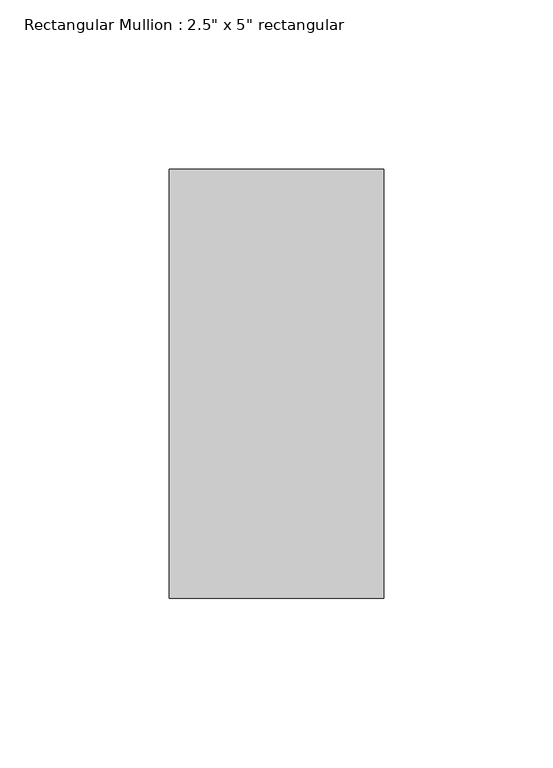
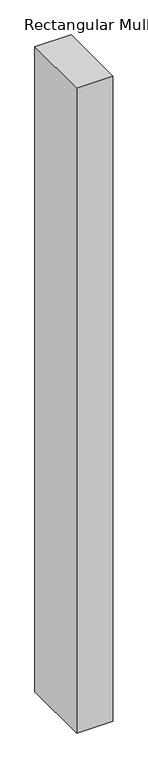
"""IFC4 building model written with IfcOpenShell, lengths in millimetres: member geometry."""

from ifc_helpers import new_model, si_unit, frame, origin, place, context, project, spatial, polyline, outline, extrude, source, transform, mapped, element, save


def member_24c95a33(model_context):
    return source(origin(), model_context, "Body", "SweptSolid", [
        extrude(outline(polyline([(0.0, 63.5), (0.0, -63.5), (-63.5, -63.5), (-63.5, 63.5), (0.0, 63.5)])), frame((0.0, 0.0, -1194.1019988), z_axis=(0.0, 0.0, 1.0), x_axis=(1.0, 0.0, 0.0)), (0.0, 0.0, 1.0), 1194.1019988),
    ])


if __name__ == "__main__":
    model = new_model("IFC4")
    model_context = context("Model", 3, world=origin())
    ifc_project = project(units=[si_unit("LENGTHUNIT", "METRE", prefix="MILLI")], contexts=[model_context])
    site = spatial("IfcSite", under=ifc_project)
    building = spatial("IfcBuilding", under=site)
    placement = place(None, origin())
    member_shape = member_24c95a33(model_context)
    element("IfcMember", 1, ObjectType="Rectangular Mullion : 2.5\" x 5\" rectangular", at=placement, inside=building, context=model_context, shape_type="MappedRepresentation", body=[
        mapped(member_shape, transform((0.0, 0.0, 0.0), x_axis=(1.0, 0.0, 0.0), y_axis=(0.0, 1.0, 0.0), z_axis=(0.0, 0.0, 1.0))),
    ])
    save(model, "model.ifc")

# Revit data of these elements
# Type "Rectangular Mullion : 2.5\" x 5\" rectangular"
#   built-in parameter 1007304 = 0.416667 (stored number, unit not read)
#   built-in parameter 1007301 = 0.104167 (stored number, unit not read)
#   built-in parameter 1007300 = 0.104167 (stored number, unit not read)
# Element 1 (IfcMember, "Rectangular Mullion : 2.5\" x 5\" rectangular")
#   Materials on its faces: "Aluminum"
# Materials
#   "Aluminum": class "Metal", colour RGB 247 247 247, transparency 0, Description = "Aluminum 6061", Cost = 0
